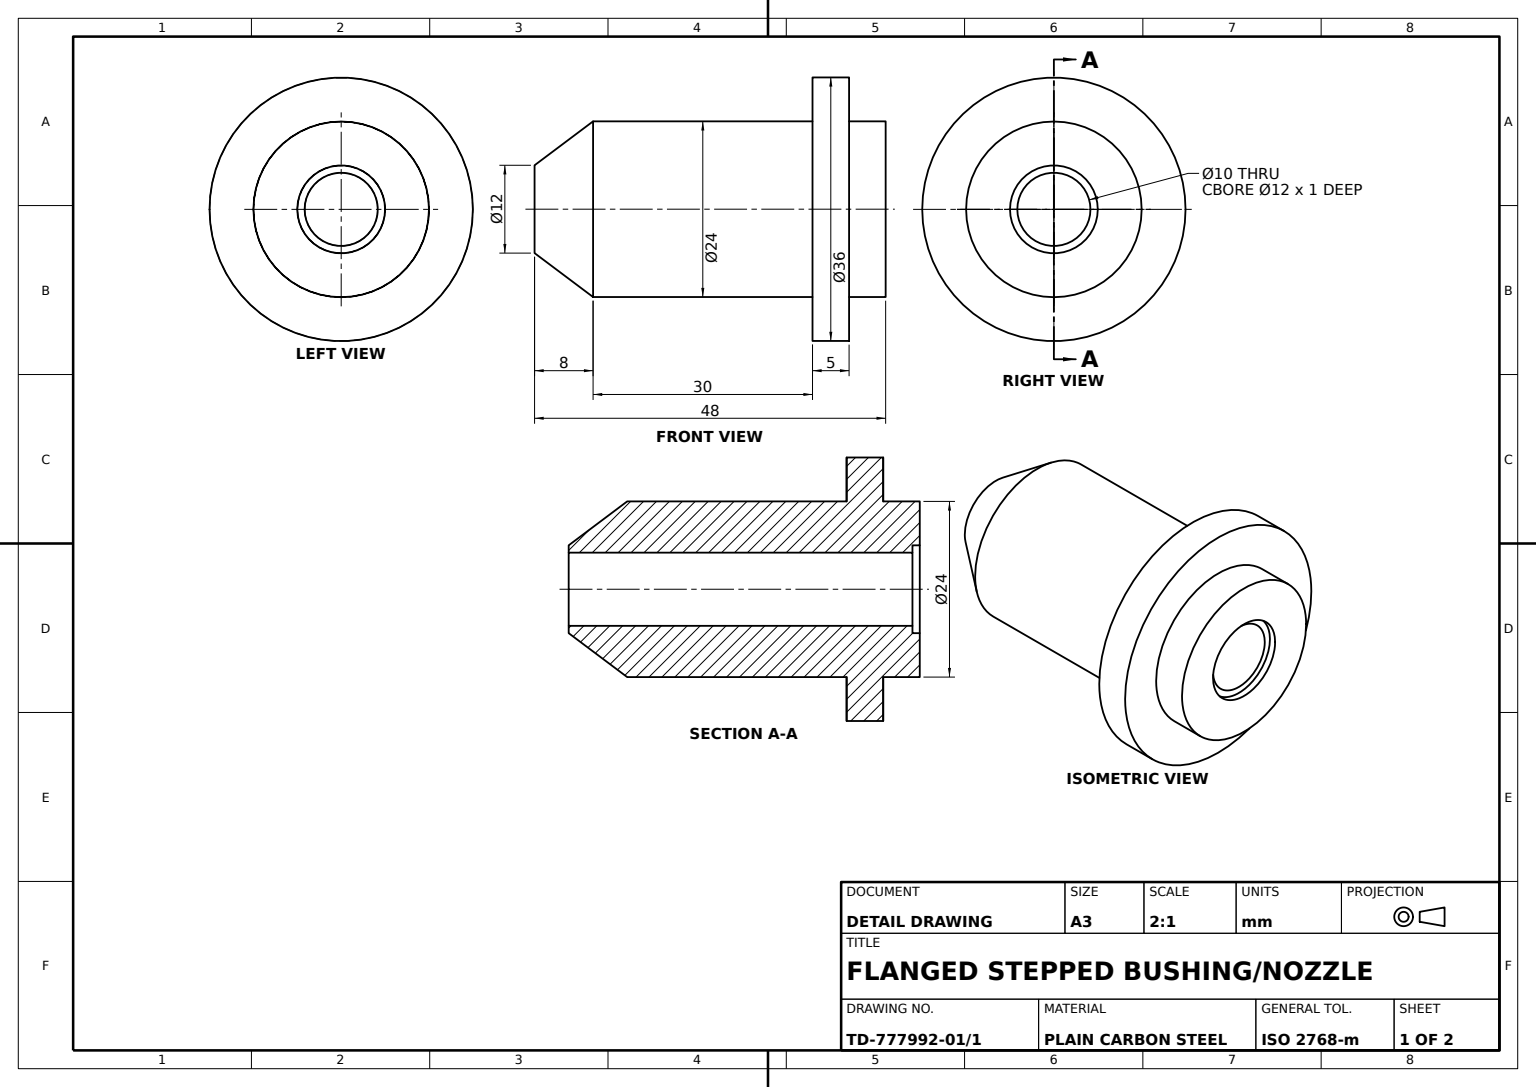
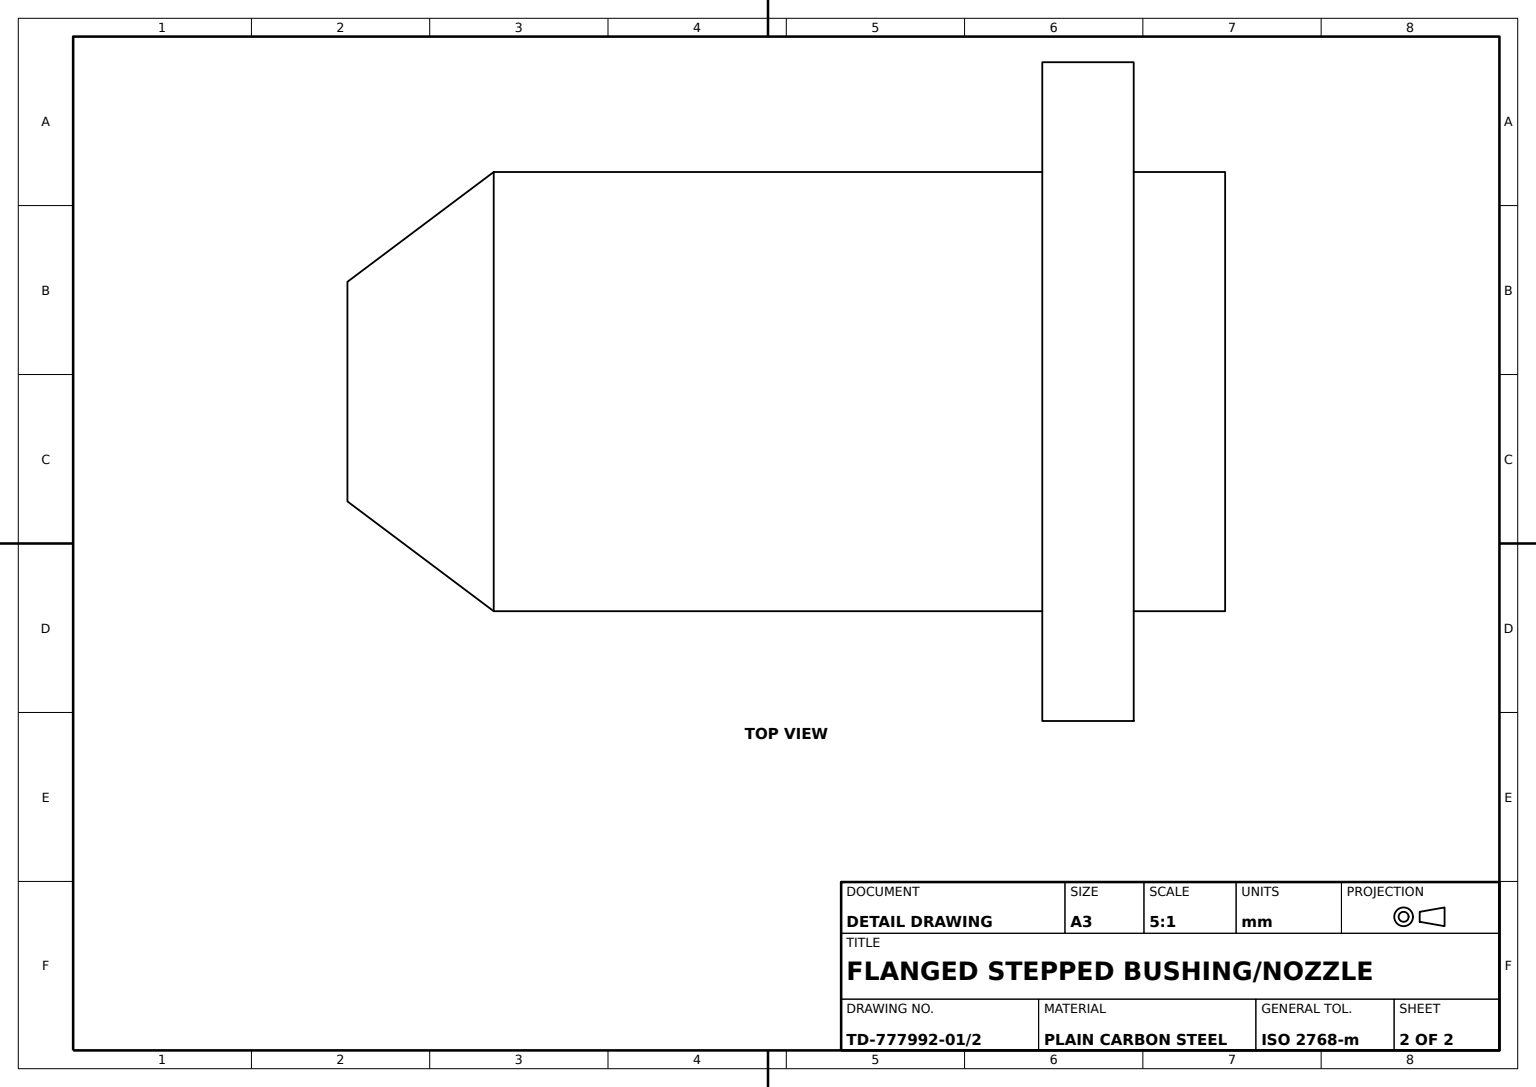
SolidWorks part; units mm, degrees
material "Plain Carbon Steel"
ref_plane "Front Plane" through (0, 0, 0) normal (0, 0, 1) x (1, 0, 0)
ref_plane "Top Plane" through (0, 0, 0) normal (0, 1, 0) x (1, 0, 0)
ref_plane "Right Plane" through (0, 0, 0) normal (1, 0, 0) x (0, 0, -1)
sketch "Nozzle Profile Sketch" plane through (0, 0, 0) normal (0, 0, 1) x (1, 0, 0)
  line L0 (0, 0) -> (0, 48) construction
  line L1 (0, 0) -> (0, 48)
  line L2 (0, 0) -> (-6, 0)
  line L3 (-12, 8) -> (-6, 0)
  line L4 (-12, 8) -> (-12, 38)
  line L5 (-12, 38) -> (-18, 38)
  line L6 (-18, 38) -> (-18, 43)
  line L7 (-18, 43) -> (-12, 43)
  line L8 (-12, 43) -> (-12, 48)
  line L9 (-12, 48) -> (0, 48)
  dimension "D1" = 8
  dimension "D2" = 48
  dimension "D3" = 6
  dimension "D4" = 12
  dimension "D5" = 5
  dimension "D6" = 30
  dimension "D7" = 6
  dimension "D8" = 6
revolve "Nozzle Body Revolve" add sketch "Nozzle Profile Sketch" angle 360 about L0
sketch "Counterbore Sketch Ø12" plane through (0, 48, 0) normal (0, 1, 0) x (1, 0, 0)
  circle A0 centre (0, 0) radius 6
  dimension "D1" = 12
extrude "Counterbore Ø12x1" cut sketch "Counterbore Sketch Ø12" against normal blind 1
sketch "Bore Sketch Ø10" plane through (0, 47, 0) normal (0, 1, 0) x (1, 0, 0)
  circle A0 centre (0, 0) radius 5
  dimension "D1" = 10
extrude "Bore Ø10x47" cut sketch "Bore Sketch Ø10" against normal blind 47
